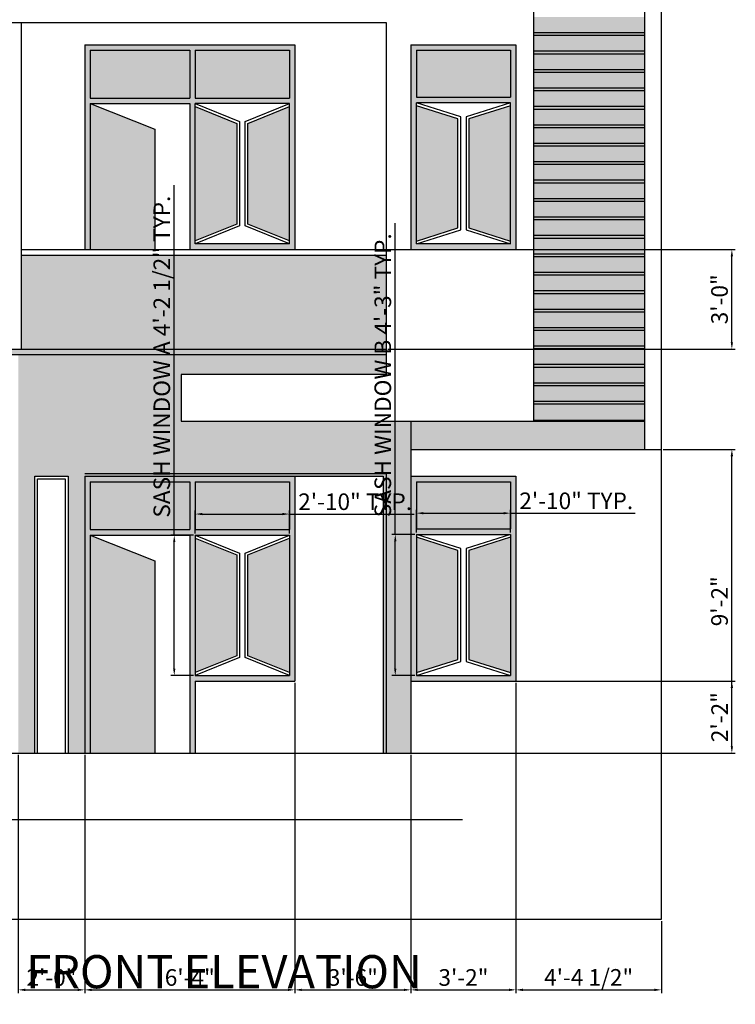
# Model space of a CAD drawing. Units: millimetres. Extents: x 67033 to 68301, y 155969 to 157209.
# Tile 8 of 17: x 68034 to 68293, y 155969 to 156325. Entities that reach past the tile are written whole.
import ezdxf

# ---------------------------------------------------------------- set-up
doc = ezdxf.new("R2010")
doc.units = ezdxf.units.MM
for name, color, linetype, lineweight in [('A-ANNO-DIMS', 2, 'Continuous', 18), ('A-AREA-IDEN', 3, 'Continuous', 18), ('A-ELEV', 7, 'Continuous', 25), ('A-ELEV-PATT', 252, 'Continuous', 13)]:
    doc.layers.add(name, color=color, linetype=linetype, lineweight=lineweight)
doc.styles.get("Standard").update_dxf_attribs({"font": 'arial.ttf'})
doc.dimstyles.new('ISO-25', dxfattribs={"dimtxt": 6, "dimasz": 2.5, "dimexe": 1.25, "dimexo": 0.625, "dimtad": 1, "dimdec": 0, "dimlunit": 3, "dimtxsty": 'Standard', "dimcen": 2.5, "dimadec": 0, "dimazin": 0, "dimtfac": 1, "dimtdec": 0, "dimtmove": 0, "dimatfit": 3, "dimfxl": 1, "dimarcsym": 0})

# ---------------------------------------------------------------- blocks, each defined once
blk = doc.blocks.new('WIN-ELEV-SASH-A')
for p, q in [((0, 50.72), (34, 50.72)), ((0, 50.72), (0, 0)), ((34, 50.72), (34, 0)), ((0, 0), (34, 0))]:
    blk.add_line(p, q)
for points in [[(0, 50.72), (16, 44.23), (16, 6.49), (0, 0)], [(34, 0), (18, 6.49), (18, 44.23), (34, 50.72)]]:
    blk.add_lwpolyline(points)
blk = doc.blocks.new('WIN-ELEV-SASH-B')
for p, q in [((0, 51), (34, 51)), ((0, 51), (0, 0)), ((34, 51), (34, 0)), ((0, 0), (34, 0))]:
    blk.add_line(p, q)
for points in [[(0, 0), (16, 5.07), (16, 45.93), (0, 51)], [(34, 51), (18, 45.93), (18, 5.07), (34, 0)]]:
    blk.add_lwpolyline(points)
blk = doc.blocks.new('*D73')
at = {"layer": 'A-ANNO-DIMS', "color": 0, "lineweight": -2, "transparency": 16777216}
for p, q in [((68090.08, 156139), (68090.08, 156265.45)), ((68097.07, 156139), (68088.83, 156139)), ((68090.08, 156090.78), (68090.08, 156136.5)), ((68097.07, 156088.28), (68088.83, 156088.28))]:
    blk.add_line(p, q, dxfattribs=at)
at = {"layer": 'A-ANNO-DIMS', "color": 0, "transparency": 16777216}
for points in [[(68089.67, 156136.5), (68090.5, 156136.5), (68090.08, 156139)], [(68089.67, 156090.78), (68090.5, 156090.78), (68090.08, 156088.28)]]:
    blk.add_solid(points, dxfattribs=at)
at = {"layer": 'Defpoints', "color": 0, "transparency": 16777216}
for p in [(68090.08, 156139), (68097.69, 156139), (68097.69, 156088.28)]:
    blk.add_point(p, dxfattribs=at)
at = {"layer": 'A-ANNO-DIMS', "color": 0, "transparency": 16777216, "insert": (68086.35, 156203.47), "char_height": 6, "attachment_point": 5, "rotation": 90}
blk.add_mtext('SASH WINDOW A 4\'-2 1/2" TYP.', dxfattribs=at)
blk = doc.blocks.new('*D74')
at = {"layer": 'A-ANNO-DIMS', "color": 0, "lineweight": -2, "transparency": 16777216}
for p, q in [((68097.69, 156139.62), (68097.69, 156147.85)), ((68131.69, 156139.62), (68131.69, 156147.85)), ((68100.19, 156146.6), (68129.19, 156146.6)), ((68131.69, 156146.6), (68176.78, 156146.6))]:
    blk.add_line(p, q, dxfattribs=at)
at = {"layer": 'A-ANNO-DIMS', "color": 0, "transparency": 16777216}
for points in [[(68100.19, 156147.02), (68100.19, 156146.19), (68097.69, 156146.6)], [(68129.19, 156147.02), (68129.19, 156146.19), (68131.69, 156146.6)]]:
    blk.add_solid(points, dxfattribs=at)
at = {"layer": 'Defpoints', "color": 0, "transparency": 16777216}
for p in [(68131.69, 156146.6), (68097.69, 156139), (68131.69, 156139)]:
    blk.add_point(p, dxfattribs=at)
at = {"layer": 'A-ANNO-DIMS', "color": 0, "transparency": 16777216, "insert": (68155.48, 156150.29), "char_height": 6, "attachment_point": 5}
blk.add_mtext('2\'-10" TYP.', dxfattribs=at)
blk = doc.blocks.new('*D75')
at = {"layer": 'A-ANNO-DIMS', "color": 0, "lineweight": -2, "transparency": 16777216}
for p, q in [((68169.99, 156139.28), (68169.99, 156251.75)), ((68177.01, 156139.28), (68168.74, 156139.28)), ((68169.99, 156090.78), (68169.99, 156136.78)), ((68177.01, 156088.28), (68168.74, 156088.28))]:
    blk.add_line(p, q, dxfattribs=at)
at = {"layer": 'A-ANNO-DIMS', "color": 0, "transparency": 16777216}
for points in [[(68169.57, 156136.78), (68170.4, 156136.78), (68169.99, 156139.28)], [(68169.57, 156090.78), (68170.4, 156090.78), (68169.99, 156088.28)]]:
    blk.add_solid(points, dxfattribs=at)
at = {"layer": 'Defpoints', "color": 0, "transparency": 16777216}
for p in [(68169.99, 156139.28), (68177.64, 156139.28), (68177.64, 156088.28)]:
    blk.add_point(p, dxfattribs=at)
at = {"layer": 'A-ANNO-DIMS', "color": 0, "transparency": 16777216, "insert": (68166.26, 156196.76), "char_height": 6, "attachment_point": 5, "rotation": 90}
blk.add_mtext('SASH WINDOW B 4\'-3" TYP.', dxfattribs=at)
blk = doc.blocks.new('*D76')
at = {"layer": 'A-ANNO-DIMS', "color": 0, "lineweight": -2, "transparency": 16777216}
for p, q in [((68177.64, 156139.9), (68177.64, 156148.18)), ((68211.64, 156139.9), (68211.64, 156148.18)), ((68180.14, 156146.93), (68209.14, 156146.93)), ((68211.64, 156146.93), (68256.73, 156146.93))]:
    blk.add_line(p, q, dxfattribs=at)
at = {"layer": 'A-ANNO-DIMS', "color": 0, "transparency": 16777216}
for points in [[(68180.14, 156147.34), (68180.14, 156146.51), (68177.64, 156146.93)], [(68209.14, 156147.34), (68209.14, 156146.51), (68211.64, 156146.93)]]:
    blk.add_solid(points, dxfattribs=at)
at = {"layer": 'Defpoints', "color": 0, "transparency": 16777216}
for p in [(68211.64, 156146.93), (68177.64, 156139.28), (68211.64, 156139.28)]:
    blk.add_point(p, dxfattribs=at)
at = {"layer": 'A-ANNO-DIMS', "color": 0, "transparency": 16777216, "insert": (68235.43, 156150.62), "char_height": 6, "attachment_point": 5}
blk.add_mtext('2\'-10" TYP.', dxfattribs=at)
blk = doc.blocks.new('*D131')
at = {"layer": 'A-ANNO-DIMS', "color": 0, "lineweight": -2, "transparency": 16777216}
for p, q in [((68033.69, 156059.57), (68033.69, 155973.45)), ((68057.69, 156059.57), (68057.69, 155973.45)), ((68036.19, 155974.7), (68055.19, 155974.7))]:
    blk.add_line(p, q, dxfattribs=at)
at = {"layer": 'A-ANNO-DIMS', "color": 0, "transparency": 16777216}
for points in [[(68036.19, 155975.12), (68036.19, 155974.28), (68033.69, 155974.7)], [(68055.19, 155975.12), (68055.19, 155974.28), (68057.69, 155974.7)]]:
    blk.add_solid(points, dxfattribs=at)
at = {"layer": 'Defpoints', "color": 0, "transparency": 16777216}
for p in [(68033.69, 156060.2), (68057.69, 156060.2), (68057.69, 155974.7)]:
    blk.add_point(p, dxfattribs=at)
at = {"layer": 'A-ANNO-DIMS', "color": 0, "transparency": 16777216, "insert": (68045.69, 155978.39), "char_height": 6, "attachment_point": 5}
blk.add_mtext('2\'-0"', dxfattribs=at)
blk = doc.blocks.new('*D132')
at = {"layer": 'A-ANNO-DIMS', "color": 0, "lineweight": -2, "transparency": 16777216}
for p, q in [((68133.69, 156085.65), (68133.69, 155973.45)), ((68057.69, 156059.57), (68057.69, 155973.45)), ((68060.19, 155974.7), (68131.19, 155974.7))]:
    blk.add_line(p, q, dxfattribs=at)
at = {"layer": 'A-ANNO-DIMS', "color": 0, "transparency": 16777216}
for points in [[(68060.19, 155975.12), (68060.19, 155974.28), (68057.69, 155974.7)], [(68131.19, 155975.12), (68131.19, 155974.28), (68133.69, 155974.7)]]:
    blk.add_solid(points, dxfattribs=at)
at = {"layer": 'Defpoints', "color": 0, "transparency": 16777216}
for p in [(68133.69, 156086.28), (68057.69, 156060.2), (68133.69, 155974.7)]:
    blk.add_point(p, dxfattribs=at)
at = {"layer": 'A-ANNO-DIMS', "color": 0, "transparency": 16777216, "insert": (68095.69, 155978.39), "char_height": 6, "attachment_point": 5}
blk.add_mtext('6\'-4"', dxfattribs=at)
blk = doc.blocks.new('*D133')
at = {"layer": 'A-ANNO-DIMS', "color": 0, "lineweight": -2, "transparency": 16777216}
for p, q in [((68133.69, 156085.65), (68133.69, 155973.45)), ((68175.64, 156059.57), (68175.64, 155973.45)), ((68136.19, 155974.7), (68173.14, 155974.7))]:
    blk.add_line(p, q, dxfattribs=at)
at = {"layer": 'A-ANNO-DIMS', "color": 0, "transparency": 16777216}
for points in [[(68136.19, 155975.12), (68136.19, 155974.28), (68133.69, 155974.7)], [(68173.14, 155975.12), (68173.14, 155974.28), (68175.64, 155974.7)]]:
    blk.add_solid(points, dxfattribs=at)
at = {"layer": 'Defpoints', "color": 0, "transparency": 16777216}
for p in [(68133.69, 156086.28), (68175.64, 156060.2), (68175.64, 155974.7)]:
    blk.add_point(p, dxfattribs=at)
at = {"layer": 'A-ANNO-DIMS', "color": 0, "transparency": 16777216, "insert": (68154.66, 155978.39), "char_height": 6, "attachment_point": 5}
blk.add_mtext('3\'-6"', dxfattribs=at)
blk = doc.blocks.new('*D134')
at = {"layer": 'A-ANNO-DIMS', "color": 0, "lineweight": -2, "transparency": 16777216}
for p, q in [((68213.64, 156085.65), (68213.64, 155973.45)), ((68175.64, 156059.57), (68175.64, 155973.45)), ((68178.14, 155974.7), (68211.14, 155974.7))]:
    blk.add_line(p, q, dxfattribs=at)
at = {"layer": 'A-ANNO-DIMS', "color": 0, "transparency": 16777216}
for points in [[(68178.14, 155975.12), (68178.14, 155974.28), (68175.64, 155974.7)], [(68211.14, 155975.12), (68211.14, 155974.28), (68213.64, 155974.7)]]:
    blk.add_solid(points, dxfattribs=at)
at = {"layer": 'Defpoints', "color": 0, "transparency": 16777216}
for p in [(68213.64, 156086.28), (68175.64, 156060.2), (68213.64, 155974.7)]:
    blk.add_point(p, dxfattribs=at)
at = {"layer": 'A-ANNO-DIMS', "color": 0, "transparency": 16777216, "insert": (68194.64, 155978.39), "char_height": 6, "attachment_point": 5}
blk.add_mtext('3\'-2"', dxfattribs=at)
blk = doc.blocks.new('*D135')
at = {"layer": 'A-ANNO-DIMS', "color": 0, "lineweight": -2, "transparency": 16777216}
for p, q in [((68213.64, 156085.65), (68213.64, 155973.45)), ((68266.19, 155999.57), (68266.19, 155973.45)), ((68216.14, 155974.7), (68263.69, 155974.7))]:
    blk.add_line(p, q, dxfattribs=at)
at = {"layer": 'A-ANNO-DIMS', "color": 0, "transparency": 16777216}
for points in [[(68216.14, 155975.12), (68216.14, 155974.28), (68213.64, 155974.7)], [(68263.69, 155975.12), (68263.69, 155974.28), (68266.19, 155974.7)]]:
    blk.add_solid(points, dxfattribs=at)
at = {"layer": 'Defpoints', "color": 0, "transparency": 16777216}
for p in [(68213.64, 156086.28), (68266.19, 156000.2), (68266.19, 155974.7)]:
    blk.add_point(p, dxfattribs=at)
at = {"layer": 'A-ANNO-DIMS', "color": 0, "transparency": 16777216, "insert": (68239.91, 155978.43), "char_height": 6, "attachment_point": 5}
blk.add_mtext('4\'-4 1/2"', dxfattribs=at)
blk = doc.blocks.new('*D141')
at = {"layer": 'A-ANNO-DIMS', "color": 0, "lineweight": -2, "transparency": 16777216}
for p, q in [((68266.82, 156169.99), (68292.94, 156169.99)), ((68291.69, 156062.7), (68291.69, 156167.49)), ((68266.82, 156060.2), (68292.94, 156060.2))]:
    blk.add_line(p, q, dxfattribs=at)
at = {"layer": 'A-ANNO-DIMS', "color": 0, "transparency": 16777216}
for points in [[(68291.27, 156167.49), (68292.11, 156167.49), (68291.69, 156169.99)], [(68291.27, 156062.7), (68292.11, 156062.7), (68291.69, 156060.2)]]:
    blk.add_solid(points, dxfattribs=at)
at = {"layer": 'Defpoints', "color": 0, "transparency": 16777216}
for p in [(68266.19, 156169.99), (68291.69, 156169.99), (68266.19, 156060.2)]:
    blk.add_point(p, dxfattribs=at)
at = {"layer": 'A-ANNO-DIMS', "color": 0, "transparency": 16777216, "insert": (68288, 156115.1), "char_height": 6, "attachment_point": 5, "rotation": 90}
blk.add_mtext('9\'-2"', dxfattribs=at)
blk = doc.blocks.new('*D147')
at = {"layer": 'A-ANNO-DIMS', "color": 0, "lineweight": -2, "transparency": 16777216}
for p, q in [((68176.26, 156086.28), (68292.94, 156086.28)), ((68291.69, 156062.7), (68291.69, 156083.78)), ((68176.26, 156060.2), (68292.94, 156060.2))]:
    blk.add_line(p, q, dxfattribs=at)
at = {"layer": 'A-ANNO-DIMS', "color": 0, "transparency": 16777216}
for points in [[(68291.27, 156083.78), (68292.11, 156083.78), (68291.69, 156086.28)], [(68291.27, 156062.7), (68292.11, 156062.7), (68291.69, 156060.2)]]:
    blk.add_solid(points, dxfattribs=at)
at = {"layer": 'Defpoints', "color": 0, "transparency": 16777216}
for p in [(68175.64, 156086.28), (68291.69, 156086.28), (68175.64, 156060.2)]:
    blk.add_point(p, dxfattribs=at)
at = {"layer": 'A-ANNO-DIMS', "color": 0, "transparency": 16777216, "insert": (68288.05, 156073.24), "char_height": 6, "attachment_point": 5, "rotation": 90}
blk.add_mtext('2\'-2"', dxfattribs=at)
blk = doc.blocks.new('*D148')
at = {"layer": 'A-ANNO-DIMS', "color": 0, "lineweight": -2, "transparency": 16777216}
for p, q in [((68134.32, 156242.2), (68292.94, 156242.2)), ((68291.69, 156208.7), (68291.69, 156239.7)), ((68167.26, 156206.2), (68292.94, 156206.2))]:
    blk.add_line(p, q, dxfattribs=at)
at = {"layer": 'A-ANNO-DIMS', "color": 0, "transparency": 16777216}
for points in [[(68291.27, 156239.7), (68292.11, 156239.7), (68291.69, 156242.2)], [(68291.27, 156208.7), (68292.11, 156208.7), (68291.69, 156206.2)]]:
    blk.add_solid(points, dxfattribs=at)
at = {"layer": 'Defpoints', "color": 0, "transparency": 16777216}
for p in [(68133.69, 156242.2), (68291.69, 156242.2), (68166.64, 156206.2)]:
    blk.add_point(p, dxfattribs=at)
at = {"layer": 'A-ANNO-DIMS', "color": 0, "transparency": 16777216, "insert": (68288, 156224.2), "char_height": 6, "attachment_point": 5, "rotation": 90}
blk.add_mtext('3\'-0"', dxfattribs=at)

msp = doc.modelspace()

# ---------------------------------------------------------------- hatches: boundary and pattern name
at = {"layer": 'A-ELEV-PATT'}
h = msp.add_hatch(color=256, dxfattribs=at)
h.dxf.hatch_style = 1
h.paths.add_polyline_path([(68260.19, 156326.25), (68219.91, 156326.25), (68219.91, 156320.59), (68260.19, 156320.59)])
h = msp.add_hatch(color=256, dxfattribs=at)
h.dxf.hatch_style = 1
h.paths.add_polyline_path([(68260.19, 156320.59), (68219.91, 156320.59), (68219.91, 156319.59), (68260.19, 156319.59)])
h = msp.add_hatch(color=256, dxfattribs=at)
h.dxf.hatch_style = 1
h.paths.add_polyline_path([(68260.19, 156319.59), (68219.91, 156319.59), (68219.91, 156313.93), (68260.19, 156313.93)])
h = msp.add_hatch(color=256, dxfattribs=at)
h.dxf.hatch_style = 1
h.paths.add_polyline_path([(68133.69, 156316.2), (68057.69, 156316.2), (68057.69, 156242.2), (68059.69, 156242.2), (68059.69, 156294.92), (68095.69, 156294.92), (68095.69, 156242.2), (68133.69, 156242.2)])
h.paths.add_polyline_path([(68097.69, 156244.2), (68097.69, 156294.92), (68131.69, 156294.92), (68131.69, 156244.2)], flags=16)
h.paths.add_polyline_path([(68097.69, 156296.92), (68097.69, 156314.2), (68131.69, 156314.2), (68131.69, 156296.92)], flags=16)
h.paths.add_polyline_path([(68095.69, 156296.92), (68059.69, 156296.92), (68059.69, 156314.2), (68095.69, 156314.2)], flags=16)
h = msp.add_hatch(color=256, dxfattribs=at)
h.dxf.hatch_style = 1
h.paths.add_polyline_path([(68213.64, 156316.2), (68175.64, 156316.2), (68175.64, 156242.2), (68213.64, 156242.2)])
h.paths.add_polyline_path([(68177.64, 156244.2), (68177.64, 156295.2), (68211.64, 156295.2), (68211.64, 156244.2)], flags=16)
h.paths.add_polyline_path([(68177.64, 156297.2), (68177.64, 156314.2), (68211.64, 156314.2), (68211.64, 156297.2)], flags=16)
h = msp.add_hatch(color=256, dxfattribs=at)
h.dxf.hatch_style = 1
h.paths.add_polyline_path([(68095.69, 156314.2), (68059.69, 156314.2), (68059.69, 156296.92), (68095.69, 156296.92)])
h = msp.add_hatch(color=256, dxfattribs=at)
h.dxf.hatch_style = 1
h.paths.add_polyline_path([(68131.69, 156314.2), (68097.69, 156314.2), (68097.69, 156296.92), (68131.69, 156296.92)])
h = msp.add_hatch(color=256, dxfattribs=at)
h.dxf.hatch_style = 1
h.paths.add_polyline_path([(68211.64, 156314.2), (68177.64, 156314.2), (68177.64, 156297.2), (68211.64, 156297.2)])
h = msp.add_hatch(color=256, dxfattribs=at)
h.dxf.hatch_style = 1
h.paths.add_polyline_path([(68260.19, 156313.93), (68219.91, 156313.93), (68219.91, 156312.93), (68260.19, 156312.93)])
h = msp.add_hatch(color=256, dxfattribs=at)
h.dxf.hatch_style = 1
h.paths.add_polyline_path([(68260.19, 156312.93), (68219.91, 156312.93), (68219.91, 156307.27), (68260.19, 156307.27)])
h = msp.add_hatch(color=256, dxfattribs=at)
h.dxf.hatch_style = 1
h.paths.add_polyline_path([(68260.19, 156307.27), (68219.91, 156307.27), (68219.91, 156306.27), (68260.19, 156306.27)])
h = msp.add_hatch(color=256, dxfattribs=at)
h.dxf.hatch_style = 1
h.paths.add_polyline_path([(68260.19, 156306.27), (68219.91, 156306.27), (68219.91, 156300.61), (68260.19, 156300.61)])
h = msp.add_hatch(color=256, dxfattribs=at)
h.dxf.hatch_style = 1
h.paths.add_polyline_path([(68260.19, 156300.61), (68219.91, 156300.61), (68219.91, 156299.61), (68260.19, 156299.61)])
h = msp.add_hatch(color=256, dxfattribs=at)
h.dxf.hatch_style = 1
h.paths.add_polyline_path([(68260.19, 156299.61), (68219.91, 156299.61), (68219.91, 156293.95), (68260.19, 156293.95)])
h = msp.add_hatch(color=256, dxfattribs=at)
h.dxf.hatch_style = 1
h.paths.add_polyline_path([(68083, 156285.64), (68059.69, 156294.92), (68059.69, 156242.2), (68083, 156242.2)])
h = msp.add_hatch(color=256, dxfattribs=at)
h.dxf.hatch_style = 1
h.paths.add_polyline_path([(68112.69, 156287.75), (68097.69, 156293.84), (68097.69, 156245.28), (68112.69, 156251.37)])
h = msp.add_hatch(color=256, dxfattribs=at)
h.dxf.hatch_style = 1
h.paths.add_polyline_path([(68131.69, 156293.84), (68116.69, 156287.75), (68116.69, 156251.37), (68131.69, 156245.28)])
h = msp.add_hatch(color=256, dxfattribs=at)
h.dxf.hatch_style = 1
h.paths.add_polyline_path([(68192.64, 156289.39), (68177.64, 156294.15), (68177.64, 156245.25), (68192.64, 156250.01)])
h = msp.add_hatch(color=256, dxfattribs=at)
h.dxf.hatch_style = 1
h.paths.add_polyline_path([(68211.64, 156294.15), (68196.64, 156289.39), (68196.64, 156250.01), (68211.64, 156245.25)])
h = msp.add_hatch(color=256, dxfattribs=at)
h.dxf.hatch_style = 1
h.paths.add_polyline_path([(68260.19, 156293.95), (68219.91, 156293.95), (68219.91, 156292.95), (68260.19, 156292.95)])
h = msp.add_hatch(color=256, dxfattribs=at)
h.dxf.hatch_style = 1
h.paths.add_polyline_path([(68260.19, 156292.95), (68219.91, 156292.95), (68219.91, 156287.29), (68260.19, 156287.29)])
h = msp.add_hatch(color=256, dxfattribs=at)
h.dxf.hatch_style = 1
h.paths.add_polyline_path([(68260.19, 156287.29), (68219.91, 156287.29), (68219.91, 156286.29), (68260.19, 156286.29)])
h = msp.add_hatch(color=256, dxfattribs=at)
h.dxf.hatch_style = 1
h.paths.add_polyline_path([(68260.19, 156286.29), (68219.91, 156286.29), (68219.91, 156280.63), (68260.19, 156280.63)])
h = msp.add_hatch(color=256, dxfattribs=at)
h.dxf.hatch_style = 1
h.paths.add_polyline_path([(68260.19, 156280.63), (68219.91, 156280.63), (68219.91, 156279.63), (68260.19, 156279.63)])
h = msp.add_hatch(color=256, dxfattribs=at)
h.dxf.hatch_style = 1
h.paths.add_polyline_path([(68260.19, 156279.63), (68219.91, 156279.63), (68219.91, 156273.97), (68260.19, 156273.97)])
h = msp.add_hatch(color=256, dxfattribs=at)
h.dxf.hatch_style = 1
h.paths.add_polyline_path([(68260.19, 156273.97), (68219.91, 156273.97), (68219.91, 156272.97), (68260.19, 156272.97)])
h = msp.add_hatch(color=256, dxfattribs=at)
h.dxf.hatch_style = 1
h.paths.add_polyline_path([(68260.19, 156272.97), (68219.91, 156272.97), (68219.91, 156267.31), (68260.19, 156267.31)])
h = msp.add_hatch(color=256, dxfattribs=at)
h.dxf.hatch_style = 1
h.paths.add_polyline_path([(68260.19, 156267.31), (68219.91, 156267.31), (68219.91, 156266.31), (68260.19, 156266.31)])
h = msp.add_hatch(color=256, dxfattribs=at)
h.dxf.hatch_style = 1
h.paths.add_polyline_path([(68260.19, 156266.31), (68219.91, 156266.31), (68219.91, 156260.65), (68260.19, 156260.65)])
h = msp.add_hatch(color=256, dxfattribs=at)
h.dxf.hatch_style = 1
h.paths.add_polyline_path([(68260.19, 156260.65), (68219.91, 156260.65), (68219.91, 156259.65), (68260.19, 156259.65)])
h = msp.add_hatch(color=256, dxfattribs=at)
h.dxf.hatch_style = 1
h.paths.add_polyline_path([(68260.19, 156259.65), (68219.91, 156259.65), (68219.91, 156253.99), (68260.19, 156253.99)])
h = msp.add_hatch(color=256, dxfattribs=at)
h.dxf.hatch_style = 1
h.paths.add_polyline_path([(68260.19, 156253.99), (68219.91, 156253.99), (68219.91, 156252.99), (68260.19, 156252.99)])
h = msp.add_hatch(color=256, dxfattribs=at)
h.dxf.hatch_style = 1
h.paths.add_polyline_path([(68260.19, 156252.99), (68219.91, 156252.99), (68219.91, 156247.33), (68260.19, 156247.33)])
h = msp.add_hatch(color=256, dxfattribs=at)
h.dxf.hatch_style = 1
h.paths.add_polyline_path([(68260.19, 156247.33), (68219.91, 156247.33), (68219.91, 156246.33), (68260.19, 156246.33)])
h = msp.add_hatch(color=256, dxfattribs=at)
h.dxf.hatch_style = 1
h.paths.add_polyline_path([(68260.19, 156246.33), (68219.91, 156246.33), (68219.91, 156240.67), (68260.19, 156240.67)])
h = msp.add_hatch(color=256, dxfattribs=at)
h.dxf.hatch_style = 1
h.paths.add_polyline_path([(68166.64, 156240.2), (68034.69, 156240.2), (68034.69, 156206.2), (68166.64, 156206.2)])
h = msp.add_hatch(color=256, dxfattribs=at)
h.dxf.hatch_style = 1
h.paths.add_polyline_path([(68260.19, 156240.67), (68219.91, 156240.67), (68219.91, 156239.67), (68260.19, 156239.67)])
h = msp.add_hatch(color=256, dxfattribs=at)
h.dxf.hatch_style = 1
h.paths.add_polyline_path([(68260.19, 156239.67), (68219.91, 156239.67), (68219.91, 156234.01), (68260.19, 156234.01)])
h = msp.add_hatch(color=256, dxfattribs=at)
h.dxf.hatch_style = 1
h.paths.add_polyline_path([(68260.19, 156234.01), (68219.91, 156234.01), (68219.91, 156233.01), (68260.19, 156233.01)])
h = msp.add_hatch(color=256, dxfattribs=at)
h.dxf.hatch_style = 1
h.paths.add_polyline_path([(68260.19, 156233.01), (68219.91, 156233.01), (68219.91, 156227.35), (68260.19, 156227.35)])
h = msp.add_hatch(color=256, dxfattribs=at)
h.dxf.hatch_style = 1
h.paths.add_polyline_path([(68260.19, 156227.35), (68219.91, 156227.35), (68219.91, 156226.35), (68260.19, 156226.35)])
h = msp.add_hatch(color=256, dxfattribs=at)
h.dxf.hatch_style = 1
h.paths.add_polyline_path([(68260.19, 156226.35), (68219.91, 156226.35), (68219.91, 156220.69), (68260.19, 156220.69)])
h = msp.add_hatch(color=256, dxfattribs=at)
h.dxf.hatch_style = 1
h.paths.add_polyline_path([(68260.19, 156220.69), (68219.91, 156220.69), (68219.91, 156219.69), (68260.19, 156219.69)])
h = msp.add_hatch(color=256, dxfattribs=at)
h.dxf.hatch_style = 1
h.paths.add_polyline_path([(68260.19, 156219.69), (68219.91, 156219.69), (68219.91, 156214.03), (68260.19, 156214.03)])
h = msp.add_hatch(color=256, dxfattribs=at)
h.dxf.hatch_style = 1
h.paths.add_polyline_path([(68260.19, 156214.03), (68219.91, 156214.03), (68219.91, 156213.03), (68260.19, 156213.03)])
h = msp.add_hatch(color=256, dxfattribs=at)
h.dxf.hatch_style = 1
h.paths.add_polyline_path([(68260.19, 156213.03), (68219.91, 156213.03), (68219.91, 156207.37), (68260.19, 156207.37)])
h = msp.add_hatch(color=256, dxfattribs=at)
h.dxf.hatch_style = 1
h.paths.add_polyline_path([(68166.64, 156206.2), (67929.86, 156206.2), (67929.86, 156204.2), (68166.64, 156204.2)])
h = msp.add_hatch(color=256, dxfattribs=at)
h.dxf.hatch_style = 1
h.paths.add_polyline_path([(68260.19, 156207.37), (68219.91, 156207.37), (68219.91, 156206.37), (68260.19, 156206.37)])
h = msp.add_hatch(color=256, dxfattribs=at)
h.dxf.hatch_style = 1
h.paths.add_polyline_path([(68260.19, 156206.37), (68219.91, 156206.37), (68219.91, 156200.71), (68260.19, 156200.71)])
h = msp.add_hatch(color=256, dxfattribs=at)
h.dxf.hatch_style = 1
h.paths.add_polyline_path([(68175.64, 156180.2), (68092.61, 156180.2), (68092.61, 156197.05), (68166.64, 156197.05), (68166.64, 156204.2), (68033.69, 156204.2), (68033.69, 156060.2), (68039.69, 156060.2), (68039.69, 156160.28), (68051.69, 156160.28), (68051.69, 156060.2), (68057.69, 156060.2), (68057.69, 156160.28), (68133.69, 156160.28), (68165.64, 156160.28), (68165.64, 156060.2), (68175.64, 156060.2)])
h = msp.add_hatch(color=256, dxfattribs=at)
h.dxf.hatch_style = 1
h.paths.add_polyline_path([(68260.19, 156200.71), (68219.91, 156200.71), (68219.91, 156199.71), (68260.19, 156199.71)])
h = msp.add_hatch(color=256, dxfattribs=at)
h.dxf.hatch_style = 1
h.paths.add_polyline_path([(68260.19, 156199.71), (68219.91, 156199.71), (68219.91, 156194.05), (68260.19, 156194.05)])
h = msp.add_hatch(color=256, dxfattribs=at)
h.dxf.hatch_style = 1
h.paths.add_polyline_path([(68260.19, 156194.05), (68219.91, 156194.05), (68219.91, 156193.05), (68260.19, 156193.05)])
h = msp.add_hatch(color=256, dxfattribs=at)
h.dxf.hatch_style = 1
h.paths.add_polyline_path([(68260.19, 156193.05), (68219.91, 156193.05), (68219.91, 156187.39), (68260.19, 156187.39)])
h = msp.add_hatch(color=256, dxfattribs=at)
h.dxf.hatch_style = 1
h.paths.add_polyline_path([(68260.19, 156187.39), (68219.91, 156187.39), (68219.91, 156186.39), (68260.19, 156186.39)])
h = msp.add_hatch(color=256, dxfattribs=at)
h.dxf.hatch_style = 1
h.paths.add_polyline_path([(68260.19, 156186.39), (68219.91, 156186.39), (68219.91, 156180.53), (68260.19, 156180.53)])
h = msp.add_hatch(color=256, dxfattribs=at)
h.dxf.hatch_style = 1
h.paths.add_polyline_path([(68260.19, 156180.2), (68175.64, 156180.2), (68175.64, 156169.99), (68260.19, 156169.99)])
h = msp.add_hatch(color=256, dxfattribs=at)
h.dxf.hatch_style = 1
h.paths.add_polyline_path([(68133.69, 156160.28), (68057.69, 156160.28), (68057.69, 156060.2), (68059.69, 156060.2), (68059.69, 156139), (68095.69, 156139), (68095.69, 156060.2), (68097.69, 156060.2), (68097.69, 156086.28), (68133.69, 156086.28)])
h.paths.add_polyline_path([(68095.69, 156158.28), (68095.69, 156141), (68059.69, 156141), (68059.69, 156158.28)], flags=16)
h.paths.add_polyline_path([(68097.69, 156158.28), (68131.69, 156158.28), (68131.69, 156141), (68097.69, 156141)], flags=16)
h.paths.add_polyline_path([(68097.69, 156139), (68131.69, 156139), (68131.69, 156088.28), (68097.69, 156088.28)], flags=16)
h = msp.add_hatch(color=256, dxfattribs=at)
h.dxf.hatch_style = 1
h.paths.add_polyline_path([(68095.69, 156158.28), (68059.69, 156158.28), (68059.69, 156141), (68095.69, 156141)])
h = msp.add_hatch(color=256, dxfattribs=at)
h.dxf.hatch_style = 1
h.paths.add_polyline_path([(68131.69, 156158.28), (68097.69, 156158.28), (68097.69, 156141), (68131.69, 156141)])
h = msp.add_hatch(color=256, dxfattribs=at)
h.dxf.hatch_style = 1
h.paths.add_polyline_path([(68213.64, 156160.28), (68175.64, 156160.28), (68175.64, 156086.28), (68213.64, 156086.28)])
h.paths.add_polyline_path([(68177.64, 156088.28), (68177.64, 156139.28), (68211.64, 156139.28), (68211.64, 156088.28)], flags=16)
h.paths.add_polyline_path([(68177.64, 156141.28), (68177.64, 156158.28), (68211.64, 156158.28), (68211.64, 156141.28)], flags=16)
h = msp.add_hatch(color=256, dxfattribs=at)
h.dxf.hatch_style = 1
h.paths.add_polyline_path([(68211.64, 156158.28), (68177.64, 156158.28), (68177.64, 156141.28), (68211.64, 156141.28)])
h = msp.add_hatch(color=256, dxfattribs=at)
h.dxf.hatch_style = 1
h.paths.add_polyline_path([(68083, 156129.71), (68059.69, 156139), (68059.69, 156060.2), (68083, 156060.2)])
h = msp.add_hatch(color=256, dxfattribs=at)
h.dxf.hatch_style = 1
h.paths.add_polyline_path([(68112.69, 156131.83), (68097.69, 156137.92), (68097.69, 156089.36), (68112.69, 156095.44)])
h = msp.add_hatch(color=256, dxfattribs=at)
h.dxf.hatch_style = 1
h.paths.add_polyline_path([(68131.69, 156137.92), (68116.69, 156131.83), (68116.69, 156095.44), (68131.69, 156089.36)])
h = msp.add_hatch(color=256, dxfattribs=at)
h.dxf.hatch_style = 1
h.paths.add_polyline_path([(68192.64, 156133.47), (68177.64, 156138.23), (68177.64, 156089.33), (68192.64, 156094.08)])
h = msp.add_hatch(color=256, dxfattribs=at)
h.dxf.hatch_style = 1
h.paths.add_polyline_path([(68211.64, 156138.23), (68196.64, 156133.47), (68196.64, 156094.08), (68211.64, 156089.33)])

# ---------------------------------------------------------------- linework, layer by layer
at = {"layer": 'A-ELEV'}
for p, q in [((68266.19, 156000.2), (68266.19, 156418.2)), ((68260.19, 156169.99), (68260.19, 156412.2)), ((68219.91, 156350.2), (68219.91, 156180.2)), ((67927.19, 156324.2), (68166.64, 156324.2)), ((68034.69, 156324.2), (68034.69, 156206.2)), ((68166.64, 156324.2), (68166.64, 156197.05)), ((68219.91, 156320.59), (68260.19, 156320.59)), ((68219.91, 156319.59), (68260.19, 156319.59)), ((68057.69, 156316.2), (68057.69, 156242.2)), ((68057.69, 156316.2), (68133.69, 156316.2)), ((68133.69, 156316.2), (68133.69, 156242.2)), ((68175.64, 156316.2), (68213.64, 156316.2)), ((68175.64, 156316.2), (68175.64, 156242.2)), ((68213.64, 156316.2), (68213.64, 156242.2)), ((68059.69, 156314.2), (68059.69, 156296.92)), ((68059.69, 156314.2), (68095.69, 156314.2)), ((68095.69, 156314.2), (68095.69, 156296.92)), ((68097.69, 156314.2), (68097.69, 156296.92)), ((68097.69, 156314.2), (68131.69, 156314.2)), ((68131.69, 156314.2), (68131.69, 156296.92)), ((68177.64, 156314.2), (68177.64, 156297.2)), ((68177.64, 156314.2), (68211.64, 156314.2)), ((68211.64, 156314.2), (68211.64, 156297.2)), ((68219.91, 156313.93), (68260.19, 156313.93)), ((68219.91, 156312.93), (68260.19, 156312.93)), ((68219.91, 156307.27), (68260.19, 156307.27)), ((68219.91, 156306.27), (68260.19, 156306.27)), ((68219.91, 156300.61), (68260.19, 156300.61)), ((68059.69, 156296.92), (68095.69, 156296.92)), ((68097.69, 156296.92), (68131.69, 156296.92)), ((68177.64, 156297.2), (68211.64, 156297.2)), ((68219.91, 156299.61), (68260.19, 156299.61)), ((68059.69, 156294.92), (68059.69, 156242.2)), ((68059.69, 156294.92), (68095.69, 156294.92)), ((68059.69, 156294.92), (68083, 156285.64)), ((68095.69, 156294.92), (68095.69, 156242.2)), ((68219.91, 156293.95), (68260.19, 156293.95)), ((68219.91, 156292.95), (68260.19, 156292.95)), ((68219.91, 156287.29), (68260.19, 156287.29)), ((68219.91, 156286.29), (68260.19, 156286.29)), ((68083, 156285.64), (68083, 156242.2)), ((68219.91, 156280.63), (68260.19, 156280.63)), ((68219.91, 156279.63), (68260.19, 156279.63)), ((68219.91, 156273.97), (68260.19, 156273.97)), ((68219.91, 156272.97), (68260.19, 156272.97)), ((68219.91, 156267.31), (68260.19, 156267.31)), ((68219.91, 156266.31), (68260.19, 156266.31)), ((68219.91, 156260.65), (68260.19, 156260.65)), ((68219.91, 156259.65), (68260.19, 156259.65)), ((68219.91, 156253.99), (68260.19, 156253.99)), ((68219.91, 156252.99), (68260.19, 156252.99)), ((68219.91, 156247.33), (68260.19, 156247.33)), ((68219.91, 156246.33), (68260.19, 156246.33)), ((68034.69, 156242.2), (68166.64, 156242.2)), ((68034.69, 156240.2), (68166.64, 156240.2)), ((68175.64, 156242.2), (68213.64, 156242.2)), ((68219.91, 156240.67), (68260.19, 156240.67)), ((68219.91, 156239.67), (68260.19, 156239.67)), ((68219.91, 156234.01), (68260.19, 156234.01)), ((68219.91, 156233.01), (68260.19, 156233.01)), ((68219.91, 156227.35), (68260.19, 156227.35)), ((68219.91, 156226.35), (68260.19, 156226.35)), ((68219.91, 156220.69), (68260.19, 156220.69)), ((68219.91, 156219.69), (68260.19, 156219.69)), ((68219.91, 156214.03), (68260.19, 156214.03)), ((68219.91, 156213.03), (68260.19, 156213.03)), ((67929.86, 156206.2), (68166.64, 156206.2)), ((68219.91, 156207.37), (68260.19, 156207.37)), ((68219.91, 156206.37), (68260.19, 156206.37)), ((67929.86, 156204.2), (68166.64, 156204.2)), ((68219.91, 156200.71), (68260.19, 156200.71)), ((68219.91, 156199.71), (68260.19, 156199.71)), ((68166.64, 156197.05), (68092.61, 156197.05)), ((68092.61, 156197.05), (68092.61, 156180.2)), ((68219.91, 156194.05), (68260.19, 156194.05)), ((68219.91, 156193.05), (68260.19, 156193.05)), ((68219.91, 156187.39), (68260.19, 156187.39)), ((68219.91, 156186.39), (68260.19, 156186.39)), ((68092.61, 156180.2), (68260.19, 156180.2)), ((68175.64, 156180.2), (68175.64, 156060.2)), ((68219.91, 156180.53), (68260.19, 156180.53)), ((68175.64, 156169.99), (68266.19, 156169.99)), ((68057.69, 156161.28), (68166.64, 156161.28)), ((68057.69, 156160.28), (68057.69, 156060.2)), ((68057.69, 156160.28), (68133.69, 156160.28)), ((68059.69, 156158.28), (68059.69, 156141)), ((68059.69, 156158.28), (68095.69, 156158.28)), ((68095.69, 156158.28), (68095.69, 156141)), ((68097.69, 156158.28), (68097.69, 156141)), ((68097.69, 156158.28), (68131.69, 156158.28)), ((68131.69, 156158.28), (68131.69, 156141)), ((68133.69, 156160.28), (68133.69, 156086.28)), ((68133.69, 156160.28), (68165.64, 156160.28)), ((68165.64, 156160.28), (68165.64, 156060.2)), ((68166.64, 156161.28), (68166.64, 156060.2)), ((68175.64, 156160.28), (68213.64, 156160.28)), ((68177.64, 156158.28), (68211.64, 156158.28)), ((68177.64, 156158.28), (68177.64, 156141.28)), ((68211.64, 156158.28), (68211.64, 156141.28)), ((68213.64, 156160.28), (68213.64, 156086.28)), ((68059.69, 156141), (68095.69, 156141)), ((68097.69, 156141), (68131.69, 156141)), ((68177.64, 156141.28), (68211.64, 156141.28)), ((68059.69, 156139), (68095.69, 156139)), ((68059.69, 156139), (68059.69, 156060.2)), ((68059.69, 156139), (68083, 156129.71)), ((68095.69, 156139), (68095.69, 156060.2)), ((68083, 156129.71), (68083, 156060.2)), ((68097.69, 156086.28), (68133.69, 156086.28)), ((68097.69, 156086.28), (68097.69, 156060.2)), ((68175.64, 156086.28), (68213.64, 156086.28)), ((67931.69, 156060.2), (68266.19, 156060.2)), ((68004.58, 156036.2), (68194.31, 156036.2)), ((67927.19, 156000.2), (68266.19, 156000.2))]:
    msp.add_line(p, q, dxfattribs=at)
for points in [[(68097.69, 156293.84), (68112.69, 156287.75), (68112.69, 156251.37), (68097.69, 156245.28)], [(68131.69, 156245.28), (68116.69, 156251.37), (68116.69, 156287.75), (68131.69, 156293.84)], [(68177.64, 156245.25), (68192.64, 156250.01), (68192.64, 156289.39), (68177.64, 156294.15)], [(68211.64, 156294.15), (68196.64, 156289.39), (68196.64, 156250.01), (68211.64, 156245.25)], [(68039.69, 156060.2), (68039.69, 156160.28), (68051.69, 156160.28), (68051.69, 156060.2)], [(68040.69, 156060.2), (68040.69, 156159.28), (68050.69, 156159.28), (68050.69, 156060.2)], [(68097.69, 156137.92), (68112.69, 156131.83), (68112.69, 156095.44), (68097.69, 156089.36)], [(68131.69, 156089.36), (68116.69, 156095.44), (68116.69, 156131.83), (68131.69, 156137.92)], [(68177.64, 156089.33), (68192.64, 156094.08), (68192.64, 156133.47), (68177.64, 156138.23)], [(68211.64, 156138.23), (68196.64, 156133.47), (68196.64, 156094.08), (68211.64, 156089.33)]]:
    msp.add_lwpolyline(points, dxfattribs=at)

# ---------------------------------------------------------------- block references
at = {"layer": 'A-ELEV', "rotation": 180}
for name, p in [('WIN-ELEV-SASH-A', (68131.69, 156294.92)), ('WIN-ELEV-SASH-B', (68211.64, 156295.2))]:
    msp.add_blockref(name, p, dxfattribs=at)
at = {"layer": 'A-ELEV'}
for name, p in [('WIN-ELEV-SASH-A', (68097.69, 156088.28)), ('WIN-ELEV-SASH-B', (68177.64, 156088.28))]:
    msp.add_blockref(name, p, dxfattribs=at)

# ---------------------------------------------------------------- texts
at = {"layer": 'A-AREA-IDEN', "insert": (68036.55, 155987.26), "char_height": 12, "attachment_point": 1}
msp.add_mtext_dynamic_manual_height_columns('FRONT ELEVATION', width=203.6887, gutter_width=12.5, heights=[0], dxfattribs=at)

# ---------------------------------------------------------------- dimensions: what is measured, and where the dimension line sits
at = {"layer": 'A-ANNO-DIMS'}
for base, p1, p2, text, picture, middle in [((68090.08, 156139), (68097.69, 156088.28), (68097.69, 156139), 'SASH WINDOW A <> TYP.', '*D73', (68086.35, 156203.47)), ((68169.99, 156139.28), (68177.64, 156088.28), (68177.64, 156139.28), 'SASH WINDOW B <> TYP.', '*D75', (68166.26, 156196.76))]:
    dim = msp.add_linear_dim(base=base, p1=p1, p2=p2, angle=90, text=text, dimstyle='ISO-25', override={"dimdec": 1, "dimrnd": 0, "dimzin": 1, "dimlunit": 4, "dimfrac": 2}, dxfattribs=at)
    dim.commit()
    dim.dimension.update_dxf_attribs({"geometry": picture, "text_midpoint": middle})
for base, p1, p2, picture, middle in [((68291.69, 156242.2), (68166.64, 156206.2), (68133.69, 156242.2), '*D148', (68288, 156224.2)), ((68291.69, 156169.99), (68266.19, 156060.2), (68266.19, 156169.99), '*D141', (68288, 156115.1)), ((68291.69, 156086.28), (68175.64, 156060.2), (68175.64, 156086.28), '*D147', (68288.05, 156073.24))]:
    dim = msp.add_linear_dim(base=base, p1=p1, p2=p2, angle=90, dimstyle='ISO-25', override={"dimdec": 1, "dimlfac": 1, "dimrnd": 0, "dimzin": 1, "dimdsep": 46, "dimlunit": 4, "dimfrac": 2}, dxfattribs=at)
    dim.commit()
    dim.dimension.update_dxf_attribs({"geometry": picture, "text_midpoint": middle})
for base, p1, p2, picture, middle in [((68131.69, 156146.6), (68097.69, 156139), (68131.69, 156139), '*D74', (68155.48, 156150.29)), ((68211.64, 156146.93), (68177.64, 156139.28), (68211.64, 156139.28), '*D76', (68235.43, 156150.62))]:
    dim = msp.add_linear_dim(base=base, p1=p1, p2=p2, text='<> TYP.', dimstyle='ISO-25', override={"dimdec": 1, "dimrnd": 0, "dimzin": 1, "dimlunit": 4, "dimfrac": 2}, dxfattribs=at)
    dim.commit()
    dim.dimension.update_dxf_attribs({"geometry": picture, "text_midpoint": middle})
for base, p1, p2, picture, middle in [((68133.69, 155974.7), (68057.69, 156060.2), (68133.69, 156086.28), '*D132', (68095.69, 155978.39)), ((68175.6382, 155974.6997), (68133.6909, 156086.2772), (68175.6382, 156060.1997), '*D133', (68154.6646, 155978.3902)), ((68213.64, 155974.7), (68175.64, 156060.2), (68213.64, 156086.28), '*D134', (68194.64, 155978.39)), ((68266.1909, 155974.6997), (68213.6382, 156086.2772), (68266.1909, 156000.1997), '*D135', (68239.9146, 155978.427)), ((68057.69, 155974.7), (68033.69, 156060.2), (68057.69, 156060.2), '*D131', (68045.69, 155978.39))]:
    dim = msp.add_linear_dim(base=base, p1=p1, p2=p2, dimstyle='ISO-25', override={"dimdec": 1, "dimlfac": 1, "dimrnd": 0, "dimzin": 1, "dimdsep": 46, "dimlunit": 4, "dimfrac": 2}, dxfattribs=at)
    dim.commit()
    dim.dimension.update_dxf_attribs({"geometry": picture, "text_midpoint": middle})

doc.saveas('drawing.dxf')
